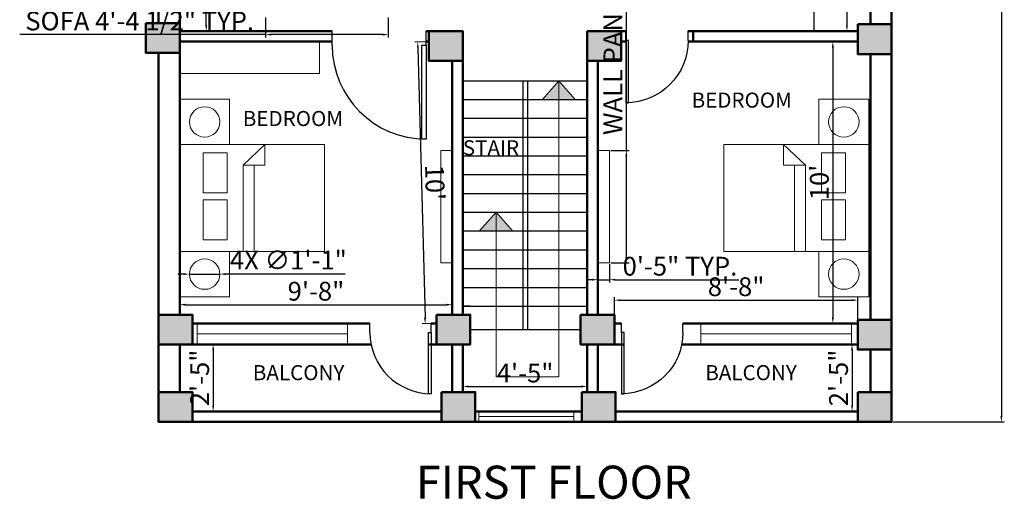
# Model space of a CAD drawing. Units: inches. Extents: x 716 to 1282, y 805 to 1949.
# Tile 1 of 2: x 716 to 1135, y 805 to 1009. Entities that reach past the tile are written whole.
import ezdxf

# ---------------------------------------------------------------- set-up
doc = ezdxf.new("R2010")
doc.units = ezdxf.units.IN
for name, color, linetype, lineweight in [('A-ANNO-DIMS', 2, 'Continuous', 18), ('A-ANNO-SYMB', 10, 'Continuous', 18), ('A-ANNO-TEXT', 10, 'Continuous', 35), ('A-AREA-IDEN', 10, 'Continuous', 25), ('A-COLS', 7, 'Continuous', 50), ('A-COLS-PATT', 252, 'Continuous', 13), ('A-DOOR', 3, 'Continuous', 25), ('A-FLOR-CASE', 32, 'Continuous', 25), ('A-FLOR-STRS', 7, 'Continuous', 25), ('A-FURN', 8, 'Continuous', 18), ('A-GLAZ', 4, 'Continuous', 18), ('WALL', 150, 'Continuous', 50)]:
    doc.layers.add(name, color=color, linetype=linetype, lineweight=lineweight)
doc.styles.get("Standard").update_dxf_attribs({"font": 'arial.ttf'})
doc.dimstyles.new('ISO-25', dxfattribs={"dimtxt": 8, "dimasz": 2.5, "dimexe": 1.25, "dimexo": 0.625, "dimtad": 1, "dimdec": 0, "dimlunit": 4, "dimtxsty": 'Standard', "dimcen": 2.5, "dimadec": 0, "dimazin": 0, "dimtfac": 1, "dimtdec": 0, "dimtmove": 0, "dimatfit": 3, "dimfxl": 1, "dimarcsym": 0})

# ---------------------------------------------------------------- blocks, each defined once
blk = doc.blocks.new('*U2')
for p, q in [((0, 0), (0, -6)), ((40, 0), (40, -6))]:
    blk.add_line(p, q)
blk.add_lwpolyline([(0, 0), (0, 40), (1.75, 40), (1.75, 0)], close=True)
blk.add_arc((0, 0), 40, 0, 90)
blk = doc.blocks.new('*D6')
at = {"layer": 'A-ANNO-DIMS', "color": 0, "lineweight": -2, "transparency": 16777216}
for p, q in [((1088.02, 1257.69), (1135.39, 1257.69)), ((1134.14, 1255.19), (1134.14, 840.19)), ((1088.02, 837.69), (1135.39, 837.69))]:
    blk.add_line(p, q, dxfattribs=at)
at = {"layer": 'A-ANNO-DIMS', "color": 0, "transparency": 16777216}
for points in [[(1133.72, 1255.19), (1134.55, 1255.19), (1134.14, 1257.69)], [(1133.72, 840.19), (1134.55, 840.19), (1134.14, 837.69)]]:
    blk.add_solid(points, dxfattribs=at)
at = {"layer": 'Defpoints', "color": 0, "transparency": 16777216}
for p in [(1087.39, 1257.69), (1087.39, 837.69), (1134.14, 837.69)]:
    blk.add_point(p, dxfattribs=at)
at = {"layer": 'A-ANNO-DIMS', "color": 0, "transparency": 16777216, "insert": (1129.42, 1047.69), "char_height": 8, "attachment_point": 5, "rotation": 90}
blk.add_mtext("35'", dxfattribs=at)
blk = doc.blocks.new('*D16')
at = {"layer": 'A-ANNO-DIMS', "color": 0, "lineweight": -2, "transparency": 16777216}
for p, q in [((1072.37, 1100.19), (1067.14, 1100.19)), ((1068.39, 1097.69), (1068.39, 1006.69)), ((1072.37, 1004.19), (1067.14, 1004.19))]:
    blk.add_line(p, q, dxfattribs=at)
at = {"layer": 'A-ANNO-DIMS', "color": 0, "transparency": 16777216}
for points in [[(1067.97, 1097.69), (1068.8, 1097.69), (1068.39, 1100.19)], [(1067.97, 1006.69), (1068.8, 1006.69), (1068.39, 1004.19)]]:
    blk.add_solid(points, dxfattribs=at)
at = {"layer": 'Defpoints', "color": 0, "transparency": 16777216}
for p in [(1072.99, 1100.19), (1068.39, 1004.19), (1072.99, 1004.19)]:
    blk.add_point(p, dxfattribs=at)
at = {"layer": 'A-ANNO-DIMS', "color": 0, "transparency": 16777216, "insert": (1063.68, 1052.19), "char_height": 8, "attachment_point": 5, "rotation": 90}
blk.add_mtext("8'", dxfattribs=at)
blk = doc.blocks.new('*D17')
at = {"layer": 'A-ANNO-DIMS', "color": 0, "lineweight": -2, "transparency": 16777216}
for p, q in [((1072.37, 999.69), (1061.14, 999.69)), ((1062.39, 997.19), (1062.39, 882.19)), ((1072.37, 879.69), (1061.14, 879.69))]:
    blk.add_line(p, q, dxfattribs=at)
at = {"layer": 'A-ANNO-DIMS', "color": 0, "transparency": 16777216}
for points in [[(1061.98, 997.19), (1062.81, 997.19), (1062.39, 999.69)], [(1061.98, 882.19), (1062.81, 882.19), (1062.39, 879.69)]]:
    blk.add_solid(points, dxfattribs=at)
at = {"layer": 'Defpoints', "color": 0, "transparency": 16777216}
for p in [(1072.99, 999.69), (1062.39, 879.69), (1072.99, 879.69)]:
    blk.add_point(p, dxfattribs=at)
at = {"layer": 'A-ANNO-DIMS', "color": 0, "transparency": 16777216, "insert": (1057.68, 939.69), "char_height": 8, "attachment_point": 5, "rotation": 90}
blk.add_mtext("10'", dxfattribs=at)
blk = doc.blocks.new('*D18')
at = {"layer": 'A-ANNO-DIMS', "color": 0, "lineweight": -2, "transparency": 16777216}
for p, q in [((969.44, 880.32), (969.44, 890.8)), ((971.94, 889.55), (1070.49, 889.55)), ((1072.99, 880.32), (1072.99, 890.8))]:
    blk.add_line(p, q, dxfattribs=at)
at = {"layer": 'A-ANNO-DIMS', "color": 0, "transparency": 16777216}
for points in [[(971.94, 889.97), (971.94, 889.14), (969.44, 889.55)], [(1070.49, 889.97), (1070.49, 889.14), (1072.99, 889.55)]]:
    blk.add_solid(points, dxfattribs=at)
at = {"layer": 'Defpoints', "color": 0, "transparency": 16777216}
for p in [(1072.99, 889.55), (969.44, 879.69), (1072.99, 879.69)]:
    blk.add_point(p, dxfattribs=at)
at = {"layer": 'A-ANNO-DIMS', "color": 0, "transparency": 16777216, "insert": (1021.22, 894.26), "char_height": 8, "attachment_point": 5}
blk.add_mtext('8\'-8"', dxfattribs=at)
blk = doc.blocks.new('*D19')
at = {"layer": 'A-ANNO-DIMS', "color": 0, "lineweight": -2, "transparency": 16777216}
for p, q in [((1072.37, 870.69), (1069.32, 870.69)), ((1070.57, 868.19), (1070.57, 844.69)), ((1072.37, 842.19), (1069.32, 842.19))]:
    blk.add_line(p, q, dxfattribs=at)
at = {"layer": 'A-ANNO-DIMS', "color": 0, "transparency": 16777216}
for points in [[(1070.16, 868.19), (1070.99, 868.19), (1070.57, 870.69)], [(1070.16, 844.69), (1070.99, 844.69), (1070.57, 842.19)]]:
    blk.add_solid(points, dxfattribs=at)
at = {"layer": 'Defpoints', "color": 0, "transparency": 16777216}
for p in [(1072.99, 870.69), (1070.57, 842.19), (1072.99, 842.19)]:
    blk.add_point(p, dxfattribs=at)
at = {"layer": 'A-ANNO-DIMS', "color": 0, "transparency": 16777216, "insert": (1065.86, 856.44), "char_height": 8, "attachment_point": 5, "rotation": 90}
blk.add_mtext('2\'-5"', dxfattribs=at)
blk = doc.blocks.new('*D20')
at = {"layer": 'A-ANNO-DIMS', "color": 0, "lineweight": -2, "transparency": 16777216}
for p, q in [((904.89, 851), (904.89, 854.05)), ((907.39, 852.8), (955.39, 852.8)), ((957.89, 851), (957.89, 854.05))]:
    blk.add_line(p, q, dxfattribs=at)
at = {"layer": 'A-ANNO-DIMS', "color": 0, "transparency": 16777216}
for points in [[(907.39, 853.22), (907.39, 852.39), (904.89, 852.8)], [(955.39, 853.22), (955.39, 852.39), (957.89, 852.8)]]:
    blk.add_solid(points, dxfattribs=at)
at = {"layer": 'Defpoints', "color": 0, "transparency": 16777216}
for p in [(957.89, 852.8), (904.89, 850.38), (957.89, 850.38)]:
    blk.add_point(p, dxfattribs=at)
at = {"layer": 'A-ANNO-DIMS', "color": 0, "transparency": 16777216, "insert": (931.39, 857.5), "char_height": 8, "attachment_point": 5}
blk.add_mtext('4\'-5"', dxfattribs=at)
blk = doc.blocks.new('*D21')
at = {"layer": 'A-ANNO-DIMS', "color": 0, "lineweight": -2, "transparency": 16777216}
for p, q in [((790.42, 870.69), (799.87, 870.69)), ((798.62, 868.19), (798.62, 844.69)), ((790.42, 842.19), (799.87, 842.19))]:
    blk.add_line(p, q, dxfattribs=at)
at = {"layer": 'A-ANNO-DIMS', "color": 0, "transparency": 16777216}
for points in [[(798.21, 868.19), (799.04, 868.19), (798.62, 870.69)], [(798.21, 844.69), (799.04, 844.69), (798.62, 842.19)]]:
    blk.add_solid(points, dxfattribs=at)
at = {"layer": 'Defpoints', "color": 0, "transparency": 16777216}
for p in [(789.79, 870.69), (789.79, 842.19), (798.62, 842.19)]:
    blk.add_point(p, dxfattribs=at)
at = {"layer": 'A-ANNO-DIMS', "color": 0, "transparency": 16777216, "insert": (793.92, 856.44), "char_height": 8, "attachment_point": 5, "rotation": 90}
blk.add_mtext('2\'-5"', dxfattribs=at)
blk = doc.blocks.new('*D22')
at = {"layer": 'A-ANNO-DIMS', "color": 0, "lineweight": -2, "transparency": 16777216}
for p, q in [((784.39, 884), (784.39, 888.88)), ((900.39, 884), (900.39, 888.88)), ((786.89, 887.63), (897.89, 887.63))]:
    blk.add_line(p, q, dxfattribs=at)
at = {"layer": 'A-ANNO-DIMS', "color": 0, "transparency": 16777216}
for points in [[(786.89, 888.04), (786.89, 887.21), (784.39, 887.63)], [(897.89, 888.04), (897.89, 887.21), (900.39, 887.63)]]:
    blk.add_solid(points, dxfattribs=at)
at = {"layer": 'Defpoints', "color": 0, "transparency": 16777216}
for p in [(900.39, 887.63), (784.39, 883.38), (900.39, 883.38)]:
    blk.add_point(p, dxfattribs=at)
at = {"layer": 'A-ANNO-DIMS', "color": 0, "transparency": 16777216, "insert": (842.39, 892.34), "char_height": 8, "attachment_point": 5}
blk.add_mtext('9\'-8"', dxfattribs=at)
blk = doc.blocks.new('*D23')
at = {"layer": 'A-ANNO-DIMS', "color": 0, "lineweight": -2, "transparency": 16777216}
for p, q in [((889.87, 999.67), (884.43, 999.53)), ((885.75, 997.06), (888.81, 882.06)), ((893.06, 879.67), (887.62, 879.53))]:
    blk.add_line(p, q, dxfattribs=at)
at = {"layer": 'A-ANNO-DIMS', "color": 0, "transparency": 16777216}
for points in [[(886.16, 997.08), (885.33, 997.05), (885.68, 999.56)], [(889.22, 882.07), (888.39, 882.05), (888.87, 879.56)]]:
    blk.add_solid(points, dxfattribs=at)
at = {"layer": 'Defpoints', "color": 0, "transparency": 16777216}
for p in [(890.49, 999.69), (888.87, 879.56), (893.69, 879.69)]:
    blk.add_point(p, dxfattribs=at)
at = {"layer": 'A-ANNO-DIMS', "color": 0, "transparency": 16777216, "insert": (891.98, 939.69), "char_height": 8, "attachment_point": 5, "rotation": 271.5245}
blk.add_mtext("10'", dxfattribs=at)
blk = doc.blocks.new('*D24')
at = {"layer": 'A-ANNO-DIMS', "color": 0, "lineweight": -2, "transparency": 16777216}
for p, q in [((848.65, 1100.19), (794.45, 1100.19)), ((795.7, 1006.69), (795.7, 1097.69)), ((848.65, 1004.19), (794.45, 1004.19))]:
    blk.add_line(p, q, dxfattribs=at)
at = {"layer": 'A-ANNO-DIMS', "color": 0, "transparency": 16777216}
for points in [[(795.28, 1097.69), (796.11, 1097.69), (795.7, 1100.19)], [(795.28, 1006.69), (796.11, 1006.69), (795.7, 1004.19)]]:
    blk.add_solid(points, dxfattribs=at)
at = {"layer": 'Defpoints', "color": 0, "transparency": 16777216}
for p in [(795.7, 1100.19), (849.27, 1100.19), (849.27, 1004.19)]:
    blk.add_point(p, dxfattribs=at)
at = {"layer": 'A-ANNO-DIMS', "color": 0, "transparency": 16777216, "insert": (790.99, 1052.19), "char_height": 8, "attachment_point": 5, "rotation": 90}
blk.add_mtext("8'", dxfattribs=at)
blk = doc.blocks.new('BED-DOUBLE-WITH-NIGHTSTANDS')
for p, q in [((36.29, 64.82), (27, 56.14)), ((36.29, 56.14), (36.29, 64.82)), ((27, 19.35), (27, 56.14)), ((27, 56.14), (36.29, 56.14)), ((31.64, 56.14), (31.64, 19.35))]:
    blk.add_line(p, q)
for points in [[(0, 64.82), (21.22, 64.82), (21.22, 84.17), (0, 84.17)], [(0, 64.82), (61.64, 64.82), (61.64, 19.35), (0, 19.35)], [(9.94, 44.27), (20.15, 44.27), (20.15, 61.31), (9.94, 61.31)], [(9.94, 24.34), (20.15, 24.34), (20.15, 41.38), (9.94, 41.38)], [(0, 0), (21.22, 0), (21.22, 19.35), (0, 19.35)]]:
    blk.add_lwpolyline(points, close=True)
for centre in [(10.61, 74.5), (10.61, 9.67)]:
    blk.add_circle(centre, 6.48)
blk = doc.blocks.new('WINDOW-64IN')
blk.add_line((0, 4.5), (64.04, 4.5))
blk.add_lwpolyline([(0, 9), (64.04, 9), (64.04, 0), (0, 0)], close=True)
blk = doc.blocks.new('FURN-WALL-PANEL')
blk.add_lwpolyline([(4.92, 47.91), (0, 47.91), (0, 0), (4.92, 0)], close=True)
blk = doc.blocks.new('*D33')
at = {"layer": 'A-ANNO-DIMS', "color": 0, "lineweight": -2, "transparency": 16777216}
for p, q in [((820.93, 1009.9), (820.93, 1001.44)), ((873.18, 1009.9), (873.18, 1001.44)), ((820.93, 1002.69), (716.28, 1002.69)), ((870.68, 1002.69), (823.43, 1002.69))]:
    blk.add_line(p, q, dxfattribs=at)
at = {"layer": 'A-ANNO-DIMS', "color": 0, "transparency": 16777216}
for points in [[(823.43, 1003.11), (823.43, 1002.27), (820.93, 1002.69)], [(870.68, 1003.11), (870.68, 1002.27), (873.18, 1002.69)]]:
    blk.add_solid(points, dxfattribs=at)
at = {"layer": 'Defpoints', "color": 0, "transparency": 16777216}
for p in [(820.93, 1010.53), (873.18, 1010.53), (820.93, 1002.69)]:
    blk.add_point(p, dxfattribs=at)
at = {"layer": 'A-ANNO-DIMS', "color": 0, "transparency": 16777216, "insert": (767.35, 1007.45), "char_height": 8, "attachment_point": 5}
blk.add_mtext('SOFA 4\'-4 1/2" TYP.', dxfattribs=at)
blk = doc.blocks.new('*D35')
at = {"layer": 'A-ANNO-DIMS', "color": 0, "lineweight": -2, "transparency": 16777216}
for p, q in [((974.5, 953.37), (974.5, 1079.51)), ((967.94, 953.37), (975.75, 953.37)), ((974.5, 907.97), (974.5, 950.87)), ((967.94, 905.47), (975.75, 905.47))]:
    blk.add_line(p, q, dxfattribs=at)
at = {"layer": 'A-ANNO-DIMS', "color": 0, "transparency": 16777216}
for points in [[(974.08, 950.87), (974.92, 950.87), (974.5, 953.37)], [(974.08, 907.97), (974.92, 907.97), (974.5, 905.47)]]:
    blk.add_solid(points, dxfattribs=at)
at = {"layer": 'Defpoints', "color": 0, "transparency": 16777216}
for p in [(967.31, 953.37), (974.5, 953.37), (967.31, 905.47)]:
    blk.add_point(p, dxfattribs=at)
at = {"layer": 'A-ANNO-DIMS', "color": 0, "transparency": 16777216, "insert": (969.79, 1017.69), "char_height": 8, "attachment_point": 5, "rotation": 90}
blk.add_mtext('WALL PANEL 4\'-0" TYP.', dxfattribs=at)
blk = doc.blocks.new('*D36')
at = {"layer": 'A-ANNO-DIMS', "color": 0, "lineweight": -2, "transparency": 16777216}
for p, q in [((962.39, 904.84), (962.39, 897.03)), ((967.31, 904.84), (967.31, 897.03)), ((959.89, 898.28), (957.39, 898.28)), ((962.39, 898.28), (967.31, 898.28)), ((969.81, 898.28), (1022.33, 898.28))]:
    blk.add_line(p, q, dxfattribs=at)
at = {"layer": 'A-ANNO-DIMS', "color": 0, "transparency": 16777216}
for points in [[(959.89, 898.7), (959.89, 897.86), (962.39, 898.28)], [(969.81, 898.7), (969.81, 897.86), (967.31, 898.28)]]:
    blk.add_solid(points, dxfattribs=at)
at = {"layer": 'Defpoints', "color": 0, "transparency": 16777216}
for p in [(962.39, 905.47), (967.31, 905.47), (967.31, 898.28)]:
    blk.add_point(p, dxfattribs=at)
at = {"layer": 'A-ANNO-DIMS', "color": 0, "transparency": 16777216, "insert": (997.32, 902.99), "char_height": 8, "attachment_point": 5}
blk.add_mtext('0\'-5" TYP.', dxfattribs=at)
blk = doc.blocks.new('*D41')
at = {"layer": 'A-ANNO-DIMS', "color": 0, "lineweight": -2, "transparency": 16777216}
for p, q in [((786.02, 900.67), (783.52, 900.67)), ((788.52, 900.67), (801.48, 900.67)), ((854.78, 900.67), (803.98, 900.67))]:
    blk.add_line(p, q, dxfattribs=at)
at = {"layer": 'A-ANNO-DIMS', "color": 0, "transparency": 16777216}
for points in [[(786.02, 901.08), (786.02, 900.25), (788.52, 900.67)], [(803.98, 901.08), (803.98, 900.25), (801.48, 900.67)]]:
    blk.add_solid(points, dxfattribs=at)
at = {"layer": 'Defpoints', "color": 0, "transparency": 16777216}
for p in [(788.52, 900.67), (801.48, 900.67)]:
    blk.add_point(p, dxfattribs=at)
at = {"layer": 'A-ANNO-DIMS', "color": 0, "transparency": 16777216, "insert": (830.63, 905.6), "char_height": 8, "attachment_point": 5, "rotation": 0.0034}
blk.add_mtext('4X ∅1\'-1"', dxfattribs=at)

msp = doc.modelspace()

# ---------------------------------------------------------------- hatches: boundary and pattern name
at = {"layer": 'A-ANNO-SYMB'}
h = msp.add_hatch(color=256, dxfattribs=at)
h.dxf.hatch_style = 1
h.paths.add_polyline_path([(919.02, 927.03), (912.04, 919.03), (919.02, 919.03)])
h.paths.add_polyline_path([(919.02, 927.03), (919.02, 919.03), (924.62, 919.03), (925.98, 919.03)])
h.paths.add_polyline_path([(945.77, 983.03), (945.77, 975.03), (951.38, 975.03), (952.74, 975.03)])
h.paths.add_polyline_path([(945.77, 983.03), (938.79, 975.03), (945.77, 975.03)])
at = {"layer": 'A-COLS-PATT'}
h = msp.add_hatch(color=256, dxfattribs=at)
h.dxf.hatch_style = 1
h.paths.add_polyline_path([(789.79, 1257.69), (775.39, 1257.69), (775.39, 1245.01), (789.79, 1245.01)])
h.paths.add_polyline_path([(910.54, 1257.69), (896.14, 1257.69), (896.14, 1245.01), (910.54, 1245.01)])
h.paths.add_polyline_path([(974.53, 1257.69), (960.13, 1257.69), (960.13, 1245.01), (974.53, 1245.01)])
h.paths.add_polyline_path([(1087.39, 1257.69), (1072.99, 1257.69), (1072.99, 1245.01), (1087.39, 1245.01)])
h.paths.add_polyline_path([(789.79, 1107.76), (775.39, 1107.76), (775.39, 1095.07), (789.79, 1095.07)])
h.paths.add_polyline_path([(784.39, 1007.56), (769.99, 1007.56), (769.99, 994.87), (784.39, 994.87)])
h.paths.add_polyline_path([(789.79, 883.38), (775.39, 883.38), (775.39, 870.69), (789.79, 870.69)])
h.paths.add_polyline_path([(789.79, 850.38), (775.39, 850.38), (775.39, 837.69), (789.79, 837.69)])
h.paths.add_polyline_path([(910.16, 850.38), (895.76, 850.38), (895.76, 837.69), (910.16, 837.69)])
h.paths.add_polyline_path([(908.09, 883.38), (893.69, 883.38), (893.69, 870.69), (908.09, 870.69)])
h.paths.add_polyline_path([(969.44, 883.38), (955.04, 883.38), (955.04, 870.69), (969.44, 870.69)])
h.paths.add_polyline_path([(969.95, 850.38), (955.55, 850.38), (955.55, 837.69), (969.95, 837.69)])
h.paths.add_polyline_path([(1087.39, 881.16), (1072.99, 881.16), (1072.99, 868.48), (1087.39, 868.48)])
h.paths.add_polyline_path([(1087.39, 850.38), (1072.99, 850.38), (1072.99, 837.69), (1087.39, 837.69)])
h.paths.add_polyline_path([(1087.39, 1007.07), (1072.99, 1007.07), (1072.99, 994.38), (1087.39, 994.38)])
h.paths.add_polyline_path([(972.29, 1004.19), (957.89, 1004.19), (957.89, 991.51), (972.29, 991.51)])
h.paths.add_polyline_path([(904.89, 1004.19), (890.49, 1004.19), (890.49, 991.51), (904.89, 991.51)])
h.paths.add_polyline_path([(974.58, 1112.88), (960.18, 1112.88), (960.18, 1100.19), (974.58, 1100.19)])
h.paths.add_polyline_path([(1087.39, 1107.7), (1072.99, 1107.7), (1072.99, 1095.02), (1087.39, 1095.02)])
h.paths.add_polyline_path([(910.8, 1112.82), (896.4, 1112.82), (896.4, 1100.19), (904.89, 1100.19), (910.8, 1100.19)])

# ---------------------------------------------------------------- linework, layer by layer
at = {"layer": 'A-ANNO-SYMB'}
for p, q in [((945.77, 983.03), (938.79, 975.03)), ((938.79, 975.03), (945.77, 983.03)), ((945.77, 856.95), (945.77, 983.03)), ((945.77, 983.03), (945.77, 983.03)), ((945.77, 983.03), (952.74, 975.03)), ((951.38, 975.03), (938.79, 975.03)), ((951.38, 975.03), (952.74, 975.03)), ((912.04, 919.03), (919.02, 927.03)), ((919.02, 927.03), (919.02, 856.95)), ((919.02, 927.03), (925.98, 919.03)), ((924.62, 919.03), (912.04, 919.03)), ((924.62, 919.03), (925.98, 919.03)), ((919.02, 856.95), (945.77, 856.95))]:
    msp.add_line(p, q, dxfattribs=at)
at = {"layer": 'A-COLS'}
for points in [[(769.99, 1007.56), (784.39, 1007.56), (784.39, 994.87), (769.99, 994.87)], [(1072.99, 1007.07), (1087.39, 1007.07), (1087.39, 994.38), (1072.99, 994.38)], [(890.49, 1004.19), (904.89, 1004.19), (904.89, 991.51), (890.49, 991.51)], [(957.89, 1004.19), (972.29, 1004.19), (972.29, 991.51), (957.89, 991.51)], [(775.39, 883.38), (789.79, 883.38), (789.79, 870.69), (775.39, 870.69)], [(893.69, 883.38), (908.09, 883.38), (908.09, 870.69), (893.69, 870.69)], [(955.04, 883.38), (969.44, 883.38), (969.44, 870.69), (955.04, 870.69)], [(1072.99, 881.16), (1087.39, 881.16), (1087.39, 868.48), (1072.99, 868.48)], [(775.39, 850.38), (789.79, 850.38), (789.79, 837.69), (775.39, 837.69)], [(895.76, 850.38), (910.16, 850.38), (910.16, 837.69), (895.76, 837.69)], [(955.55, 850.38), (969.95, 850.38), (969.95, 837.69), (955.55, 837.69)], [(1072.99, 850.38), (1087.39, 850.38), (1087.39, 837.69), (1072.99, 837.69)]]:
    msp.add_lwpolyline(points, close=True, dxfattribs=at)
at = {"layer": 'A-FLOR-CASE'}
for p, q in [((1054.39, 1004.19), (1054.39, 1076.19)), ((1072.99, 1004.19), (1054.39, 1004.19))]:
    msp.add_line(p, q, dxfattribs=at)
at = {"layer": 'A-FLOR-STRS'}
for p, q in [((904.89, 983.03), (957.89, 983.03)), ((930.56, 982.78), (930.56, 983.03)), ((930.56, 877.03), (930.56, 982.78)), ((932.56, 982.78), (932.56, 983.03)), ((932.56, 877.03), (932.56, 982.78)), ((904.89, 975.03), (957.89, 975.03)), ((904.89, 967.03), (957.89, 967.03)), ((904.89, 959.03), (957.89, 959.03)), ((904.89, 951.03), (957.89, 951.03)), ((904.89, 943.03), (957.89, 943.03)), ((904.89, 935.03), (957.89, 935.03)), ((904.89, 927.03), (957.89, 927.03)), ((904.89, 919.03), (957.89, 919.03)), ((904.89, 911.03), (957.89, 911.03)), ((904.89, 903.03), (957.89, 903.03)), ((904.89, 895.03), (957.89, 895.03)), ((908.09, 887.03), (904.89, 887.03)), ((904.89, 887.03), (957.89, 887.03)), ((908.09, 887.03), (955.04, 887.03)), ((908.09, 877.03), (955.04, 877.03))]:
    msp.add_line(p, q, dxfattribs=at)
at = {"layer": 'A-FURN'}
msp.add_lwpolyline([(784.39, 999.69), (843.87, 999.69), (843.87, 986.07), (784.39, 986.07)], close=True, dxfattribs=at)
at = {"layer": 'A-GLAZ'}
msp.add_line((911.74, 839.94), (952.14, 839.94), dxfattribs=at)
msp.add_lwpolyline([(911.74, 842.19), (952.14, 842.19), (952.14, 837.69), (911.74, 837.69)], close=True, dxfattribs=at)
at = {"layer": 'WALL'}
for p, q in [((775.39, 1007.56), (775.39, 1257.69)), ((1087.39, 1257.69), (1087.39, 837.69)), ((784.39, 1095.07), (784.39, 1004.19)), ((784.39, 883.38), (784.39, 1095.07)), ((1078.39, 1095.02), (1078.39, 1007.07)), ((784.39, 1004.19), (849.27, 1004.19)), ((889.27, 1004.19), (904.89, 1004.19)), ((904.89, 1004.19), (904.89, 883.38)), ((957.89, 1004.19), (957.89, 883.38)), ((974.28, 1004.19), (957.89, 1004.19)), ((1072.99, 1004.19), (1002.89, 1004.19)), ((1002.89, 1004.19), (1002.89, 999.69)), ((1007.39, 1004.19), (1072.99, 1004.19)), ((784.39, 999.69), (849.27, 999.69)), ((784.39, 999.69), (849.27, 999.69)), ((889.27, 999.69), (890.49, 999.69)), ((889.27, 999.69), (890.49, 999.69)), ((974.28, 999.69), (972.29, 999.69)), ((1002.89, 999.69), (1000.83, 999.69)), ((1002.89, 999.69), (1072.99, 999.69)), ((1072.99, 999.69), (1002.89, 999.69)), ((775.39, 837.69), (775.39, 994.87)), ((1078.39, 994.38), (1078.39, 881.16)), ((900.39, 991.51), (900.39, 883.38)), ((962.39, 991.51), (962.39, 883.38)), ((865.38, 879.69), (789.79, 879.69)), ((893.69, 879.69), (891.43, 879.69)), ((969.44, 879.69), (972.49, 879.69)), ((998.55, 879.69), (1072.99, 879.69)), ((784.39, 850.38), (784.39, 870.69)), ((865.88, 870.69), (784.39, 870.69)), ((900.39, 870.69), (890.29, 870.69)), ((900.39, 870.69), (900.39, 850.38)), ((904.89, 870.69), (904.89, 850.38)), ((957.89, 870.69), (957.89, 850.38)), ((962.39, 870.69), (973.63, 870.69)), ((962.39, 870.69), (962.39, 850.38)), ((998.04, 870.69), (1072.99, 870.69)), ((1078.39, 868.48), (1078.39, 850.38)), ((895.76, 842.19), (789.79, 842.19)), ((955.55, 842.19), (910.16, 842.19)), ((1072.99, 842.19), (969.95, 842.19)), ((1087.39, 837.69), (775.39, 837.69))]:
    msp.add_line(p, q, dxfattribs=at)
msp.add_lwpolyline([(1002.89, 1004.19), (1000.84, 1004.19), (1000.84, 1004.19), (1002.89, 1004.19)], close=True, dxfattribs=at)

# ---------------------------------------------------------------- block references
at = {"layer": 'A-DOOR', "rotation": 180}
msp.add_blockref('*U2', (889.27, 998.19), dxfattribs=at)
for p, xscale, yscale, zscale in [((974.28, 1000.21), -0.6640096988613329, 0.6640096988613329, 0.6640096988613329), ((891.43, 875.78), 0.6514123527418816, 0.6514123527418816, 0.6514123527418816), ((972.49, 875.78), -0.6514123527418816, 0.6514123527418816, 0.6514123527418816)]:
    msp.add_blockref('*U2', p, dxfattribs=dict(at, xscale=xscale, yscale=yscale, zscale=zscale))
at = {"layer": 'A-FURN'}
for name, p in [('BED-DOUBLE-WITH-NIGHTSTANDS', (784.39, 890.99)), ('FURN-WALL-PANEL', (895.47, 905.47)), ('FURN-WALL-PANEL', (962.39, 905.47))]:
    msp.add_blockref(name, p, dxfattribs=at)
at = {"layer": 'A-FURN', "extrusion": (0, 0, -1), "zscale": -1}
msp.add_blockref('BED-DOUBLE-WITH-NIGHTSTANDS', (-1077.69, 890.99), dxfattribs=at)
at = {"layer": 'A-GLAZ'}
for p in [(791.77, 870.69), (1006.27, 870.69)]:
    msp.add_blockref('WINDOW-64IN', p, dxfattribs=at)

# ---------------------------------------------------------------- texts
at = {"layer": 'A-ANNO-TEXT', "insert": (884.88, 819.07), "char_height": 14.0872, "attachment_point": 1}
msp.add_mtext_dynamic_manual_height_columns('FIRST FLOOR', width=287.7229, gutter_width=70.44, heights=[0], dxfattribs=at)
at = {"layer": 'A-AREA-IDEN', "char_height": 6.429, "attachment_point": 1}
for s, insert in [('BEDROOM', (1002.29, 977.99)), ('BEDROOM', (811.26, 970.15)), ('STAIR', (904.89, 957.69)), ('BALCONY', (815.52, 861.9)), ('BALCONY', (1008.1, 861.9))]:
    msp.add_mtext_dynamic_manual_height_columns(s, width=131.2996, gutter_width=32.14, heights=[0], dxfattribs=dict(at, insert=insert))

# ---------------------------------------------------------------- dimensions: what is measured, and where the dimension line sits
at = {"layer": 'A-ANNO-DIMS'}
for base, p1, p2, picture, middle in [((1134.14, 837.69), (1087.39, 1257.69), (1087.39, 837.69), '*D6', (1129.42, 1047.69)), ((795.7, 1100.19), (849.27, 1004.19), (849.27, 1100.19), '*D24', (790.99, 1052.19)), ((1068.39, 1004.19), (1072.99, 1100.19), (1072.99, 1004.19), '*D16', (1063.68, 1052.19)), ((1062.39, 879.69), (1072.99, 999.69), (1072.99, 879.69), '*D17', (1057.68, 939.69)), ((798.62471028, 842.19156326), (789.79096556, 870.69156326), (789.79096556, 842.19156326), '*D21', (793.91512638, 856.44156326)), ((1070.57341086, 842.19156326), (1072.99428725, 870.69156326), (1072.99428725, 842.19156326), '*D19', (1065.86382696, 856.44156326))]:
    dim = msp.add_linear_dim(base=base, p1=p1, p2=p2, angle=90, dimstyle='ISO-25', override={"dimclrd": 0, "dimclre": 0, "dimclrt": 0}, dxfattribs=at)
    dim.commit()
    dim.dimension.update_dxf_attribs({"geometry": picture, "text_midpoint": middle})
for base, p1, p2, angle, text, picture, middle in [((974.5, 953.37), (967.31, 905.47), (967.31, 953.37), 90, 'WALL PANEL <> TYP.', '*D35', (969.79, 1017.69)), ((820.9255, 1002.6901), (873.1788, 1010.5281), (820.9255, 1010.5281), 180, 'SOFA <> TYP.', '*D33', (767.3503, 1007.4543))]:
    dim = msp.add_linear_dim(base=base, p1=p1, p2=p2, angle=angle, text=text, dimstyle='ISO-25', override={"dimdec": 1, "dimlfac": 1, "dimrnd": 0, "dimzin": 1, "dimdsep": 46, "dimlunit": 4, "dimfrac": 2}, dxfattribs=at)
    dim.commit()
    dim.dimension.update_dxf_attribs({"geometry": picture, "text_midpoint": middle})
dim = msp.add_aligned_dim(p1=(890.49, 999.69), p2=(893.69, 879.69), distance=-4.82, dimstyle='ISO-25', override={"dimclrd": 0, "dimclre": 0, "dimclrt": 0}, dxfattribs=at)
dim.commit()
dim.dimension.update_dxf_attribs({"geometry": '*D23', "text_midpoint": (891.98, 939.69)})
dim = msp.add_diameter_dim_2p(p1=(788.52, 900.67), p2=(801.48, 900.67), text='4X <>', dimstyle='ISO-25', override={"dimdec": 1, "dimlfac": 1, "dimrnd": 0, "dimzin": 1, "dimdsep": 46, "dimlunit": 4, "dimfrac": 2}, dxfattribs=at)
dim.commit()
dim.dimension.update_dxf_attribs({"geometry": '*D41', "text_midpoint": (830.63, 900.67)})
dim = msp.add_linear_dim(base=(967.31, 898.28), p1=(962.39, 905.47), p2=(967.31, 905.47), text='<> TYP.', dimstyle='ISO-25', override={"dimdec": 1, "dimlfac": 1, "dimrnd": 0, "dimzin": 1, "dimdsep": 46, "dimlunit": 4, "dimfrac": 2}, dxfattribs=at)
dim.commit()
dim.dimension.update_dxf_attribs({"geometry": '*D36', "text_midpoint": (997.32, 902.99)})
for base, p1, p2, picture, middle in [((900.39, 887.63), (784.39, 883.38), (900.39, 883.38), '*D22', (842.39, 892.34)), ((1072.99, 889.55), (969.44, 879.69), (1072.99, 879.69), '*D18', (1021.22, 894.26)), ((957.89, 852.8), (904.89, 850.38), (957.89, 850.38), '*D20', (931.39, 857.5))]:
    dim = msp.add_linear_dim(base=base, p1=p1, p2=p2, dimstyle='ISO-25', override={"dimclrd": 0, "dimclre": 0, "dimclrt": 0}, dxfattribs=at)
    dim.commit()
    dim.dimension.update_dxf_attribs({"geometry": picture, "text_midpoint": middle})

doc.saveas('drawing.dxf')
